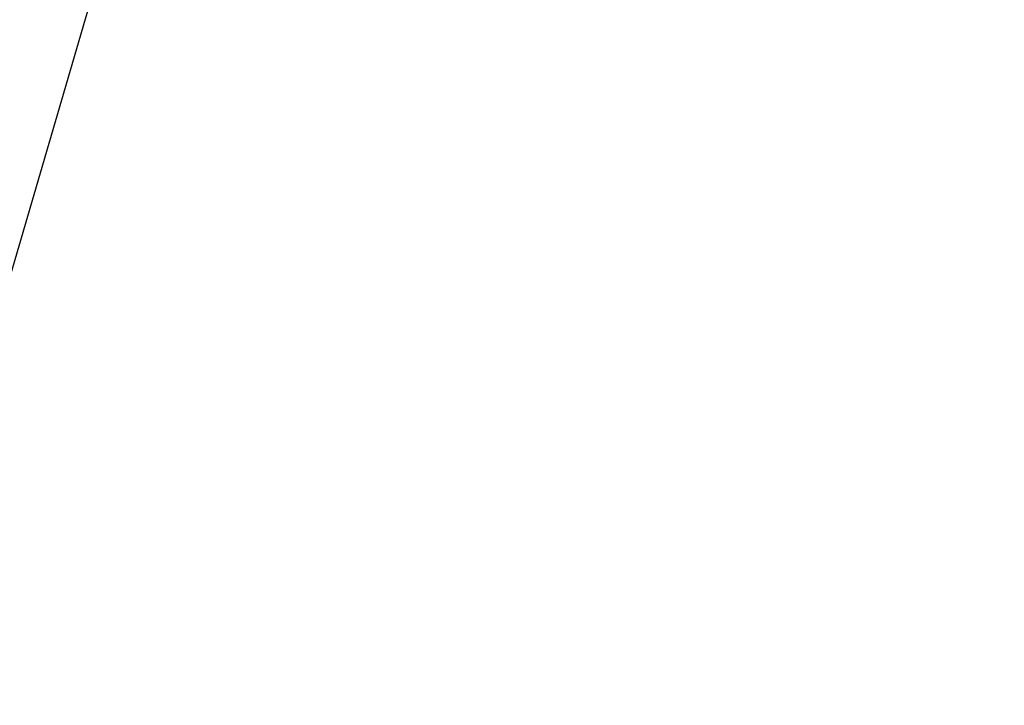
# Model space of a CAD drawing. Units: inches. Extents: x 3590 to 5167, y 65 to 1917.
# Tile 92 of 100: x 5052.8768 to 5053.476, y 1788.6144 to 1789.0318. Entities that reach past the tile are written whole.
import ezdxf

# ---------------------------------------------------------------- set-up
doc = ezdxf.new("R2010")
doc.units = ezdxf.units.IN
for name, color, linetype, lineweight in [('A-ANNO-DIMS', 2, 'Continuous', 18), ('A-FLOR-PATT', 8, 'Continuous', 13), ('L-PLNT', 94, 'Continuous', 18)]:
    doc.layers.add(name, color=color, linetype=linetype, lineweight=lineweight)
doc.layers.add('DIENHOA', color=3, linetype='Continuous')
doc.styles.get("Standard").update_dxf_attribs({"font": 'arial.ttf'})
doc.dimstyles.new('ISO-25', dxfattribs={"dimtxt": 9, "dimasz": 2.5, "dimexe": 1.25, "dimexo": 0.625, "dimtad": 1, "dimdec": 1, "dimlunit": 3, "dimtxsty": 'Standard', "dimcen": 2.5, "dimadec": 0, "dimazin": 0, "dimtfac": 1, "dimtdec": 1, "dimtmove": 0, "dimatfit": 3, "dimfxl": 1, "dimarcsym": 0})

# ---------------------------------------------------------------- blocks, each defined once
blk = doc.blocks.new('Cay03_mb')
at = {"layer": 'DIENHOA'}
blk.add_line((118.956, 441.661), (96.72, 365.576), dxfattribs=at)
blk = doc.blocks.new('*D323')
at = {"layer": 'A-ANNO-DIMS', "color": 0, "lineweight": -2, "transparency": 16777216}
for p, q in [((5069.17227, 1795.21603), (5069.17227, 1874.95034)), ((5065.43703, 1795.21603), (5070.42227, 1795.21603)), ((5069.17227, 1769.30924), (5069.17227, 1792.71603)), ((5065.43703, 1766.80924), (5070.42227, 1766.80924))]:
    blk.add_line(p, q, dxfattribs=at)
at = {"layer": 'A-ANNO-DIMS', "color": 0, "transparency": 16777216}
for points in [[(5068.75561, 1792.71603), (5069.58894, 1792.71603), (5069.17227, 1795.21603)], [(5068.75561, 1769.30924), (5069.58894, 1769.30924), (5069.17227, 1766.80924)]]:
    blk.add_solid(points, dxfattribs=at)
at = {"layer": 'Defpoints', "color": 0, "transparency": 16777216}
for p in [(5064.81203, 1795.21603), (5069.17227, 1795.21603), (5064.81203, 1766.80924)]:
    blk.add_point(p, dxfattribs=at)
at = {"layer": 'A-ANNO-DIMS', "color": 0, "transparency": 16777216, "insert": (5063.89379, 1836.33318), "char_height": 9, "attachment_point": 5, "rotation": 90}
blk.add_mtext('2\'-4 1/2" TYP.', dxfattribs=at)

msp = doc.modelspace()

# ---------------------------------------------------------------- hatches: boundary and pattern name
at = {"layer": 'A-FLOR-PATT', "transparency": 33554687}
h = msp.add_hatch(dxfattribs=at)
h.set_pattern_fill('AR-HBONE', color=256, scale=0.2)
h.set_pattern_definition([(45, (-588.972, 0), (0, 28.73682), [60.96, -20.32]), (135, (-574.604, 14.368), (3e-15, 28.73682), [60.96, -20.32])])
h.paths.add_polyline_path([(5071.27403, 1796.99898), (4933.27403, 1796.99898), (4933.27403, 1753.99898), (4962.77403, 1753.99898, -0.414214), (4928.77403, 1719.99898), (4933.27403, 1718.99898), (4933.27403, 1334.99898), (5071.27403, 1334.99898)])
h.paths.add_polyline_path([(4951.78002, 1521.0767), (4951.7151, 1521.0404), (4951.56345, 1520.89532)], flags=16)
h.paths.add_polyline_path([(4952.267, 1521.37645), (4952.1977, 1521.37111), (4952.19823, 1521.35558)], flags=0)
h.paths.add_polyline_path([(4967.05076, 1529.72832), (4965.23122, 1528.69444), (4963.41109, 1527.71401), (4961.75649, 1526.85081), (4963.58887, 1527.44938), (4964.03555, 1527.47802), (4962.9755, 1527.24902), (4961.76022, 1526.85203), (4959.79219, 1525.83406), (4958.00498, 1524.89483), (4956.24031, 1523.92961), (4954.50395, 1522.91854), (4954.1294, 1522.68163), (4953.36051, 1521.99688), (4953.36558, 1521.99754), (4953.605, 1522.06367), (4955.10605, 1522.76083), (4956.92108, 1523.43405), (4958.67784, 1523.91513), (4960.35834, 1524.20036), (4961.94456, 1524.28606), (4964.17144, 1524.10849), (4965.95752, 1523.30903), (4963.86273, 1522.97565), (4965.18742, 1522.49898), (4963.36614, 1522.49715), (4961.54526, 1522.48682), (4959.76359, 1522.46077), (4958.30414, 1522.4188), (4957.97356, 1522.38829), (4956.30692, 1522.2324), (4954.71821, 1522.07143), (4953.25077, 1521.89915), (4953.52509, 1521.62277), (4954.33087, 1521.37883), (4956.24263, 1521.22987), (4958.03913, 1520.92952), (4959.68424, 1520.48339), (4961.16007, 1519.89569), (4963.10699, 1518.80022), (4964.39286, 1517.32518), (4962.97306, 1517.72596), (4964.55841, 1516.66059), (4965.40664, 1515.70779), (4963.50733, 1516.32179), (4961.67995, 1517.0051), (4959.93478, 1517.74489), (4958.2821, 1518.52833), (4956.73216, 1519.34257), (4955.29527, 1520.17478), (4954.67155, 1520.57237), (4954.51279, 1520.6271), (4955.65848, 1519.31837), (4956.70263, 1517.98232), (4957.64403, 1516.64663), (4958.48545, 1515.33439), (4959.54998, 1513.52398), (4960.43768, 1511.76936), (4958.84107, 1513.6196), (4957.45175, 1515.3249), (4955.8186, 1517.45855), (4956.66537, 1515.44764), (4957.11109, 1513.92292), (4957.44681, 1511.71434), (4957.07641, 1509.79288), (4956.53757, 1511.1103), (4955.99231, 1512.56892), (4955.44448, 1514.12509), (4954.89794, 1515.73518), (4954.35653, 1517.35553), (4953.82412, 1518.94251), (4953.30455, 1520.45247), (4953.06452, 1521.11563), (4952.97143, 1521.14607), (4952.94932, 1521.08646), (4952.72981, 1520.19905), (4953.3698, 1518.02364), (4953.75708, 1516.37279), (4954.05124, 1514.76538), (4954.26449, 1513.22121), (4954.47124, 1511.13121), (4954.4971, 1510.40174), (4954.40903, 1511.76006), (4954.26449, 1513.22121), (4954.05124, 1514.76538), (4953.75708, 1516.37279), (4953.3698, 1518.02364), (4952.87718, 1519.69813), (4952.7161, 1520.1412), (4952.53301, 1519.05871), (4952.37428, 1517.78881), (4952.21925, 1516.31167), (4952.04598, 1514.59986), (4951.83253, 1512.62598), (4951.55697, 1510.36259), (4951.20331, 1512.16818), (4950.85168, 1514.33931), (4950.98529, 1516.37594), (4951.6596, 1518.28625), (4952.59261, 1520.48085), (4952.35664, 1521.1299), (4951.85502, 1520.32753), (4950.83901, 1518.90828), (4949.77675, 1517.58658), (4948.91554, 1516.61731), (4948.11099, 1515.2561), (4947.0891, 1513.55389), (4945.88937, 1511.61495), (4946.32587, 1513.40232), (4946.5624, 1514.24913), (4945.52771, 1513.32668), (4944.58105, 1512.53126), (4946.01774, 1514.50825), (4947.2044, 1516.04763), (4947.89331, 1517.31331), (4949.30686, 1518.76446), (4950.41417, 1519.76716), (4950.45131, 1519.80628), (4952.267, 1521.37645), (4951.64457, 1521.49317), (4950.40371, 1521.17954), (4948.04447, 1520.35868), (4946.11863, 1519.45198), (4944.57182, 1518.47484), (4943.34962, 1517.44265), (4941.99695, 1515.91971), (4941.66146, 1515.27475), (4942.81332, 1516.98973), (4944.57182, 1518.47484), (4946.11863, 1519.45198), (4948.04447, 1520.35868), (4950.40371, 1521.17954), (4951.64457, 1521.49317), (4949.64678, 1521.86781), (4948.59979, 1521.75633), (4947.12629, 1521.5699), (4945.42015, 1521.34763), (4943.44969, 1521.10462), (4941.18319, 1520.85596), (4942.86028, 1521.61265), (4943.87308, 1522.03014), (4942.95216, 1521.9093), (4941.40968, 1521.48512), (4939.54287, 1520.67019), (4938.96775, 1520.2255), (4940.73284, 1521.29899), (4942.95216, 1521.9093), (4943.70184, 1522.00767), (4945.89419, 1522.69998), (4947.56488, 1522.71399), (4948.92086, 1522.56573), (4951.13144, 1522.18271), (4950.97062, 1522.2969), (4948.12924, 1523.00563), (4946.03496, 1523.70671), (4944.23235, 1524.52143), (4942.70692, 1525.46111), (4941.44419, 1526.53707), (4940.42968, 1527.76062), (4939.6489, 1529.14306), (4941.42091, 1528.12232), (4943.14742, 1527.13248), (4944.84093, 1526.17457), (4946.51394, 1525.24959), (4948.17893, 1524.35855), (4948.36457, 1524.26336), (4946.47531, 1526.04459), (4945.18083, 1527.54042), (4944.19039, 1529.03339), (4943.49559, 1530.53985), (4943.27808, 1531.3597), (4942.49849, 1531.91903), (4943.11353, 1531.76249), (4942.95927, 1533.6586), (4944.13953, 1531.9886), (4944.61171, 1531.32339), (4946.20163, 1530.46341), (4947.48567, 1529.50925), (4948.79027, 1528.22649), (4950.36754, 1526.23746), (4949.48547, 1528.15549), (4948.85128, 1530.12254), (4948.49054, 1532.04127), (4948.38105, 1533.91822), (4948.50062, 1535.7599), (4948.82704, 1537.57284), (4949.41803, 1535.56526), (4949.95684, 1533.56932), (4950.46414, 1531.5861), (4950.96058, 1529.6167), (4951.3911, 1527.95448), (4951.72352, 1530.68689), (4952.20106, 1532.57994), (4952.88914, 1534.32964), (4953.77035, 1535.95123), (4954.82726, 1537.45995), (4954.52145, 1535.38966), (4954.27314, 1533.93684), (4955.57999, 1535.6627), (4956.74758, 1536.73859), (4956.15852, 1534.78029), (4955.58917, 1532.87334), (4955.04336, 1531.00581), (4954.52493, 1529.16576), (4954.03771, 1527.34127), (4953.63833, 1525.73298), (4953.61143, 1525.58564), (4953.39805, 1524.16565), (4953.38219, 1524.00887), (4954.06955, 1525.47563), (4954.91212, 1527.02173), (4956.13627, 1528.89351), (4957.84668, 1530.57701), (4959.37601, 1531.54014), (4958.25596, 1530.10398), (4957.14284, 1528.66291), (4956.06626, 1527.24305), (4955.05579, 1525.87054), (4954.14104, 1524.57149), (4953.35159, 1523.37204), (4953.31079, 1523.30299), (4953.27253, 1522.92478), (4953.26102, 1522.38213), (4954.1031, 1523.37273), (4954.63005, 1524.28376), (4955.96149, 1526.35767), (4957.23002, 1528.12969), (4958.42057, 1529.60864), (4960.03671, 1531.36792), (4961.3736, 1532.3752), (4962.1015, 1532.77), (4961.06994, 1531.06113), (4959.98733, 1529.43811), (4958.86851, 1527.90803), (4958.15046, 1527.00742), (4959.80291, 1528.00314), (4961.58854, 1528.79257), (4963.39087, 1529.32783), (4965.21118, 1529.63205)], flags=16)
h.paths.add_polyline_path([(4962.94387, 1523.18187), (4961.10714, 1523.42192), (4960.39205, 1523.36158), (4962.34964, 1523.33061)], flags=0)
h.paths.add_polyline_path([(5049.54129, 1584.55089), (5049.47636, 1584.51458), (5049.32471, 1584.3695)], flags=16)
h.paths.add_polyline_path([(5050.02827, 1584.85063), (5049.95897, 1584.84529), (5049.95949, 1584.82976)], flags=0)
h.paths.add_polyline_path([(5042.33308, 1581.94902), (5043.8799, 1582.92616), (5045.80573, 1583.83286), (5048.16498, 1584.65372), (5049.40583, 1584.96736), (5047.40804, 1585.34199), (5046.36106, 1585.23052), (5044.88755, 1585.04408), (5043.18142, 1584.82181), (5041.21095, 1584.5788), (5038.94446, 1584.33014), (5040.62155, 1585.08683), (5041.63434, 1585.50432), (5040.71343, 1585.38348), (5039.17095, 1584.9593), (5037.30414, 1584.14438), (5036.72901, 1583.69969), (5038.4941, 1584.77317), (5040.71343, 1585.38348), (5041.4631, 1585.48185), (5043.65545, 1586.17416), (5045.32615, 1586.18818), (5046.68212, 1586.03992), (5048.8927, 1585.6569), (5048.73188, 1585.77108), (5045.89051, 1586.47981), (5043.79622, 1587.18089), (5041.99361, 1587.99561), (5040.46818, 1588.9353), (5039.20546, 1590.01125), (5038.19095, 1591.2348), (5037.41016, 1592.61725), (5039.18217, 1591.5965), (5040.90868, 1590.60667), (5042.6022, 1589.64876), (5044.2752, 1588.72378), (5045.94019, 1587.83274), (5046.12584, 1587.73754), (5044.23658, 1589.51878), (5042.9421, 1591.01461), (5041.95166, 1592.50757), (5041.25685, 1594.01403), (5041.03935, 1594.83388), (5040.25976, 1595.39321), (5040.8748, 1595.23667), (5040.72054, 1597.13279), (5041.9008, 1595.46278), (5042.37297, 1594.79758), (5043.96289, 1593.93759), (5045.24694, 1592.98344), (5046.55153, 1591.70068), (5048.12881, 1589.71164), (5047.24673, 1591.62967), (5046.61254, 1593.59672), (5046.2518, 1595.51546), (5046.14232, 1597.3924), (5046.26189, 1599.23408), (5046.5883, 1601.04703), (5047.17929, 1599.03944), (5047.71811, 1597.0435), (5048.22541, 1595.06028), (5048.72184, 1593.09089), (5049.15237, 1591.42866), (5049.48478, 1594.16107), (5049.96233, 1596.05412), (5050.65041, 1597.80382), (5051.53161, 1599.42541), (5052.58852, 1600.93414), (5052.28271, 1598.86384), (5052.03441, 1597.41102), (5053.34126, 1599.13689), (5054.50884, 1600.21277), (5053.91979, 1598.25447), (5053.35044, 1596.34752), (5052.80463, 1594.47999), (5052.2862, 1592.63995), (5051.79898, 1590.81546), (5051.39959, 1589.20716), (5051.3727, 1589.05983), (5051.15931, 1587.63984), (5051.14346, 1587.48305), (5051.83082, 1588.94982), (5052.67339, 1590.49592), (5053.89754, 1592.3677), (5055.60794, 1594.05119), (5057.13728, 1595.01432), (5056.01722, 1593.57817), (5054.90411, 1592.1371), (5053.82752, 1590.71724), (5052.81705, 1589.34472), (5051.9023, 1588.04567), (5051.11286, 1586.84622), (5051.07205, 1586.77718), (5051.03379, 1586.39896), (5051.02228, 1585.85631), (5051.86437, 1586.84692), (5052.39131, 1587.75794), (5053.72275, 1589.83185), (5054.99128, 1591.60387), (5056.18183, 1593.08282), (5057.79798, 1594.84211), (5059.13486, 1595.84938), (5059.86276, 1596.24419), (5058.83121, 1594.53531), (5057.7486, 1592.9123), (5056.62978, 1591.38221), (5055.91173, 1590.4816), (5057.56418, 1591.47732), (5059.34981, 1592.26675), (5061.15214, 1592.80202), (5062.97245, 1593.10624), (5064.81203, 1593.20251), (5062.99248, 1592.16863), (5061.17235, 1591.18819), (5059.51775, 1590.325), (5061.35014, 1590.92356), (5061.79682, 1590.95221), (5060.73676, 1590.7232), (5059.52148, 1590.32622), (5057.55345, 1589.30825), (5055.76625, 1588.36901), (5054.00157, 1587.40379), (5052.26521, 1586.39273), (5051.89067, 1586.15581), (5051.12177, 1585.47106), (5051.12684, 1585.47172), (5051.36627, 1585.53786), (5052.86732, 1586.23502), (5054.68234, 1586.90824), (5056.4391, 1587.38931), (5058.1196, 1587.67454), (5059.70582, 1587.76024), (5061.93271, 1587.58268), (5063.71878, 1586.78321), (5061.62399, 1586.44983), (5062.94869, 1585.97317), (5061.12741, 1585.97133), (5059.30653, 1585.961), (5057.52486, 1585.93496), (5056.06541, 1585.89299), (5055.73482, 1585.86247), (5054.06819, 1585.70658), (5052.47947, 1585.54561), (5051.01204, 1585.37333), (5051.28635, 1585.09695), (5052.09214, 1584.85301), (5054.00389, 1584.70406), (5055.8004, 1584.4037), (5057.44551, 1583.95757), (5058.92133, 1583.36987), (5060.86825, 1582.27441), (5062.15413, 1580.79937), (5060.73433, 1581.20015), (5062.31967, 1580.13477), (5063.1679, 1579.18198), (5061.2686, 1579.79597), (5059.44122, 1580.47928), (5057.69605, 1581.21908), (5056.04336, 1582.00251), (5054.49343, 1582.81675), (5053.05653, 1583.64897), (5052.43281, 1584.04656), (5052.27405, 1584.10128), (5053.41974, 1582.79255), (5054.4639, 1581.4565), (5055.40529, 1580.12081), (5056.24672, 1578.80858), (5057.31125, 1576.99816), (5058.19895, 1575.24354), (5056.60234, 1577.09378), (5055.21301, 1578.79908), (5053.57987, 1580.93274), (5054.42664, 1578.92183), (5054.87235, 1577.3971), (5055.20808, 1575.18852), (5054.83767, 1573.26706), (5054.29883, 1574.58448), (5053.75357, 1576.0431), (5053.20575, 1577.59927), (5052.6592, 1579.20936), (5052.1178, 1580.82971), (5051.58538, 1582.41669), (5051.06582, 1583.92666), (5050.82578, 1584.58981), (5050.7327, 1584.62025), (5050.71058, 1584.56064), (5050.49108, 1583.67323), (5051.13107, 1581.49782), (5051.51835, 1579.84698), (5051.8125, 1578.23957), (5052.02575, 1576.69539), (5052.23251, 1574.6054), (5052.25836, 1573.87593), (5052.1703, 1575.23424), (5052.02575, 1576.69539), (5051.8125, 1578.23957), (5051.51835, 1579.84698), (5051.13107, 1581.49782), (5050.63844, 1583.17231), (5050.47736, 1583.61538), (5050.29428, 1582.53289), (5050.13554, 1581.26299), (5049.98051, 1579.78585), (5049.80724, 1578.07405), (5049.59379, 1576.10016), (5049.31823, 1573.83678), (5048.96458, 1575.64237), (5048.61294, 1577.8135), (5048.74656, 1579.85012), (5049.42086, 1581.76043), (5050.35388, 1583.95503), (5050.1179, 1584.60408), (5049.61629, 1583.80172), (5048.60027, 1582.38246), (5047.53801, 1581.06076), (5046.67681, 1580.09149), (5045.87225, 1578.73029), (5044.85036, 1577.02808), (5043.65063, 1575.08913), (5044.08713, 1576.8765), (5044.32366, 1577.72331), (5043.28898, 1576.80086), (5042.34232, 1576.00545), (5043.779, 1577.98243), (5044.96566, 1579.52182), (5045.65457, 1580.78749), (5047.06813, 1582.23865), (5048.17543, 1583.24134), (5048.21258, 1583.28047), (5050.02827, 1584.85063), (5049.40583, 1584.96736), (5048.16498, 1584.65372), (5045.80573, 1583.83286), (5043.8799, 1582.92616), (5042.33308, 1581.94902), (5041.11088, 1580.91684), (5039.75821, 1579.39389), (5039.42272, 1578.74894), (5040.57458, 1580.46391)], flags=16)
h.paths.add_polyline_path([(4954.79872, 1533.12029), (4954.26249, 1532.07935), (4953.83112, 1530.93464), (4953.50472, 1529.63602), (4953.28338, 1528.13331), (4953.16721, 1526.37637), (4953.15631, 1524.31504), (4953.27669, 1521.23629), (4952.80168, 1521.84177), (4951.55695, 1521.99789), (4950.97575, 1521.9613), (4952.66059, 1521.94097), (4952.80168, 1521.84177), (4953.15249, 1523.59258), (4953.16721, 1526.37637), (4953.28338, 1528.13331), (4953.60929, 1530.34598), (4954.45558, 1532.59174)], flags=0)
h.paths.add_polyline_path([(5050.56294, 1585.31596), (5049.31822, 1585.47208), (5048.73702, 1585.43548), (5050.42186, 1585.41516), (5050.56294, 1585.31596), (5050.91375, 1587.06676), (5050.92848, 1589.85056), (5051.04465, 1591.6075), (5051.37055, 1593.82017), (5052.21684, 1596.06593), (5052.55999, 1596.59447), (5052.02375, 1595.55353), (5051.59238, 1594.40883), (5051.26598, 1593.1102), (5051.04465, 1591.6075), (5050.92848, 1589.85056), (5050.91757, 1587.78922), (5051.03795, 1584.71048)], flags=0)
h.paths.add_polyline_path([(5058.15332, 1586.83576), (5060.11091, 1586.80479), (5060.70514, 1586.65605), (5058.8684, 1586.8961)], flags=0)
h.paths.add_polyline_path([(5049.54129, 1430.93611), (5049.47636, 1430.8998), (5049.32471, 1430.75472)], flags=16)
h.paths.add_polyline_path([(5050.02827, 1431.23585), (5049.95897, 1431.23051), (5049.95949, 1431.21498)], flags=0)
h.paths.add_polyline_path([(5046.5883, 1447.43225), (5047.17929, 1445.42467), (5047.71811, 1443.42872), (5048.22541, 1441.4455), (5048.72184, 1439.47611), (5049.15237, 1437.81388), (5049.48478, 1440.5463), (5049.96233, 1442.43934), (5050.65041, 1444.18904), (5051.53161, 1445.81063), (5052.58852, 1447.31936), (5052.28271, 1445.24906), (5052.03441, 1443.79624), (5053.34126, 1445.52211), (5054.50884, 1446.59799), (5053.91979, 1444.63969), (5053.35044, 1442.73274), (5052.80463, 1440.86521), (5052.2862, 1439.02517), (5051.79898, 1437.20068), (5051.39959, 1435.59238), (5051.3727, 1435.44505), (5051.15931, 1434.02506), (5051.14346, 1433.86828), (5051.83082, 1435.33504), (5052.67339, 1436.88114), (5053.89754, 1438.75292), (5055.60794, 1440.43641), (5057.13728, 1441.39954), (5056.01722, 1439.96339), (5054.90411, 1438.52232), (5053.82752, 1437.10246), (5052.81705, 1435.72994), (5051.9023, 1434.4309), (5051.11286, 1433.23145), (5051.07205, 1433.1624), (5051.03379, 1432.78418), (5051.02228, 1432.24153), (5051.86437, 1433.23214), (5052.39131, 1434.14316), (5053.72275, 1436.21707), (5054.99128, 1437.98909), (5056.18183, 1439.46805), (5057.79798, 1441.22733), (5059.13486, 1442.23461), (5059.86276, 1442.62941), (5058.83121, 1440.92053), (5057.7486, 1439.29752), (5056.62978, 1437.76743), (5055.91173, 1436.86682), (5057.56418, 1437.86255), (5059.34981, 1438.65197), (5061.15214, 1439.18724), (5062.97245, 1439.49146), (5064.81203, 1439.58773), (5062.99248, 1438.55385), (5061.17235, 1437.57342), (5059.51775, 1436.71022), (5061.35014, 1437.30879), (5061.79682, 1437.33743), (5060.73676, 1437.10842), (5059.52148, 1436.71144), (5057.55345, 1435.69347), (5055.76625, 1434.75423), (5054.00157, 1433.78901), (5052.26521, 1432.77795), (5051.89067, 1432.54103), (5051.12177, 1431.85628), (5051.12684, 1431.85694), (5051.36627, 1431.92308), (5052.86732, 1432.62024), (5054.68234, 1433.29346), (5056.4391, 1433.77453), (5058.1196, 1434.05976), (5059.70582, 1434.14546), (5061.93271, 1433.9679), (5063.71878, 1433.16843), (5061.62399, 1432.83505), (5062.94869, 1432.35839), (5061.12741, 1432.35655), (5059.30653, 1432.34623), (5057.52486, 1432.32018), (5056.06541, 1432.27821), (5055.73482, 1432.24769), (5054.06819, 1432.09181), (5052.47947, 1431.93083), (5051.01204, 1431.75856), (5051.28635, 1431.48218), (5052.09214, 1431.23823), (5054.00389, 1431.08928), (5055.8004, 1430.78892), (5057.44551, 1430.34279), (5058.92133, 1429.75509), (5060.86825, 1428.65963), (5062.15413, 1427.18459), (5060.73433, 1427.58537), (5062.31967, 1426.52), (5063.1679, 1425.5672), (5061.2686, 1426.18119), (5059.44122, 1426.86451), (5057.69605, 1427.6043), (5056.04336, 1428.38773), (5054.49343, 1429.20197), (5053.05653, 1430.03419), (5052.43281, 1430.43178), (5052.27405, 1430.48651), (5053.41974, 1429.17777), (5054.4639, 1427.84172), (5055.40529, 1426.50603), (5056.24672, 1425.1938), (5057.31125, 1423.38338), (5058.19895, 1421.62877), (5056.60234, 1423.479), (5055.21301, 1425.1843), (5053.57987, 1427.31796), (5054.42664, 1425.30705), (5054.87235, 1423.78233), (5055.20808, 1421.57374), (5054.83767, 1419.65228), (5054.29883, 1420.9697), (5053.75357, 1422.42832), (5053.20575, 1423.9845), (5052.6592, 1425.59458), (5052.1178, 1427.21493), (5051.58538, 1428.80191), (5051.06582, 1430.31188), (5050.82578, 1430.97503), (5050.7327, 1431.00547), (5050.71058, 1430.94586), (5050.49108, 1430.05845), (5051.13107, 1427.88305), (5051.51835, 1426.2322), (5051.8125, 1424.62479), (5052.02575, 1423.08061), (5052.23251, 1420.99062), (5052.25836, 1420.26115), (5052.1703, 1421.61947), (5052.02575, 1423.08061), (5051.8125, 1424.62479), (5051.51835, 1426.2322), (5051.13107, 1427.88305), (5050.63844, 1429.55753), (5050.47736, 1430.0006), (5050.29428, 1428.91811), (5050.13554, 1427.64821), (5049.98051, 1426.17107), (5049.80724, 1424.45927), (5049.59379, 1422.48539), (5049.31823, 1420.222), (5048.96458, 1422.02759), (5048.61294, 1424.19872), (5048.74656, 1426.23534), (5049.42086, 1428.14565), (5050.35388, 1430.34025), (5050.1179, 1430.98931), (5049.61629, 1430.18694), (5048.60027, 1428.76768), (5047.53801, 1427.44598), (5046.67681, 1426.47671), (5045.87225, 1425.11551), (5044.85036, 1423.4133), (5043.65063, 1421.47435), (5044.08713, 1423.26172), (5044.32366, 1424.10854), (5043.28898, 1423.18608), (5042.34232, 1422.39067), (5043.779, 1424.36765), (5044.96566, 1425.90704), (5045.65457, 1427.17272), (5047.06813, 1428.62387), (5048.17543, 1429.62657), (5048.21258, 1429.66569), (5050.02827, 1431.23585), (5049.40583, 1431.35258), (5048.16498, 1431.03894), (5045.80573, 1430.21809), (5043.8799, 1429.31139), (5042.33308, 1428.33424), (5041.11088, 1427.30206), (5039.75821, 1425.77911), (5039.42272, 1425.13416), (5040.57458, 1426.84914), (5042.33308, 1428.33424), (5043.8799, 1429.31139), (5045.80573, 1430.21809), (5048.16498, 1431.03894), (5049.40583, 1431.35258), (5047.40804, 1431.72722), (5046.36106, 1431.61574), (5044.88755, 1431.42931), (5043.18142, 1431.20704), (5041.21095, 1430.96402), (5038.94446, 1430.71536), (5040.62155, 1431.47205), (5041.63434, 1431.88954), (5040.71343, 1431.76871), (5039.17095, 1431.34453), (5037.30414, 1430.5296), (5036.72901, 1430.08491), (5038.4941, 1431.1584), (5040.71343, 1431.76871), (5041.4631, 1431.86707), (5043.65545, 1432.55939), (5045.32615, 1432.5734), (5046.68212, 1432.42514), (5048.8927, 1432.04212), (5048.73188, 1432.1563), (5045.89051, 1432.86503), (5043.79622, 1433.56611), (5041.99361, 1434.38083), (5040.46818, 1435.32052), (5039.20546, 1436.39648), (5038.19095, 1437.62002), (5037.41016, 1439.00247), (5039.18217, 1437.98172), (5040.90868, 1436.99189), (5042.6022, 1436.03398), (5044.2752, 1435.109), (5045.94019, 1434.21796), (5046.12584, 1434.12276), (5044.23658, 1435.904), (5042.9421, 1437.39983), (5041.95166, 1438.8928), (5041.25685, 1440.39925), (5041.03935, 1441.2191), (5040.25976, 1441.77844), (5040.8748, 1441.62189), (5040.72054, 1443.51801), (5041.9008, 1441.848), (5042.37297, 1441.1828), (5043.96289, 1440.32282), (5045.24694, 1439.36866), (5046.55153, 1438.0859), (5048.12881, 1436.09686), (5047.24673, 1438.01489), (5046.61254, 1439.98195), (5046.2518, 1441.90068), (5046.14232, 1443.77762), (5046.26189, 1445.6193)], flags=16)
h.paths.add_polyline_path([(5052.38176, 1444.25496), (5051.62263, 1442.77987), (5052.02375, 1441.93875), (5052.55999, 1442.9797)], flags=0)
h.paths.add_polyline_path([(5050.56294, 1431.70118), (5049.31822, 1431.8573), (5048.73702, 1431.82071), (5050.42186, 1431.80038)], flags=0)
h.paths.add_polyline_path([(5058.15332, 1433.22098), (5060.11091, 1433.19001), (5060.70514, 1433.04127), (5058.8684, 1433.28132)], flags=0)
h.paths.add_polyline_path([(5049.54129, 1352.28535), (5049.47636, 1352.24904), (5049.32471, 1352.10396)], flags=16)
h.paths.add_polyline_path([(5050.02827, 1352.58509), (5049.95897, 1352.57975), (5049.95949, 1352.56422)], flags=0)
h.paths.add_polyline_path([(5046.5883, 1368.78149), (5047.17929, 1366.7739), (5047.71811, 1364.77796), (5048.22541, 1362.79474), (5048.72184, 1360.82534), (5049.15237, 1359.16312), (5049.48478, 1361.89553), (5049.96233, 1363.78858), (5050.65041, 1365.53828), (5051.53161, 1367.15987), (5052.58852, 1368.6686), (5052.28271, 1366.5983), (5052.03441, 1365.14548), (5053.34126, 1366.87135), (5054.50884, 1367.94723), (5053.91979, 1365.98893), (5053.35044, 1364.08198), (5052.80463, 1362.21445), (5052.2862, 1360.37441), (5051.79898, 1358.54992), (5051.39959, 1356.94162), (5051.3727, 1356.79428), (5051.15931, 1355.37429), (5051.14346, 1355.21751), (5051.83082, 1356.68428), (5052.67339, 1358.23037), (5053.89754, 1360.10216), (5055.60794, 1361.78565), (5057.13728, 1362.74878), (5056.01722, 1361.31262), (5054.90411, 1359.87155), (5053.82752, 1358.4517), (5052.81705, 1357.07918), (5051.9023, 1355.78013), (5051.11286, 1354.58068), (5051.07205, 1354.51164), (5051.03379, 1354.13342), (5051.02228, 1353.59077), (5051.86437, 1354.58137), (5052.39131, 1355.4924), (5053.72275, 1357.56631), (5054.99128, 1359.33833), (5056.18183, 1360.81728), (5057.79798, 1362.57656), (5059.13486, 1363.58384), (5059.86276, 1363.97864), (5058.83121, 1362.26977), (5057.7486, 1360.64675), (5056.62978, 1359.11667), (5055.91173, 1358.21606), (5057.56418, 1359.21178), (5059.34981, 1360.00121), (5061.15214, 1360.53648), (5062.97245, 1360.84069), (5064.81203, 1360.93697), (5062.99248, 1359.90308), (5061.17235, 1358.92265), (5059.51775, 1358.05946), (5061.35014, 1358.65802), (5061.79682, 1358.68666), (5060.73676, 1358.45766), (5059.52148, 1358.06068), (5057.55345, 1357.0427), (5055.76625, 1356.10347), (5054.00157, 1355.13825), (5052.26521, 1354.12718), (5051.89067, 1353.89027), (5051.12177, 1353.20552), (5051.12684, 1353.20618), (5051.36627, 1353.27231), (5052.86732, 1353.96947), (5054.68234, 1354.6427), (5056.4391, 1355.12377), (5058.1196, 1355.409), (5059.70582, 1355.4947), (5061.93271, 1355.31713), (5063.71878, 1354.51767), (5061.62399, 1354.18429), (5062.94869, 1353.70763), (5061.12741, 1353.70579), (5059.30653, 1353.69546), (5057.52486, 1353.66942), (5056.06541, 1353.62744), (5055.73482, 1353.59693), (5054.06819, 1353.44104), (5052.47947, 1353.28007), (5051.01204, 1353.10779), (5051.28635, 1352.83141), (5052.09214, 1352.58747), (5054.00389, 1352.43852), (5055.8004, 1352.13816), (5057.44551, 1351.69203), (5058.92133, 1351.10433), (5060.86825, 1350.00887), (5062.15413, 1348.53382), (5060.73433, 1348.9346), (5062.31967, 1347.86923), (5063.1679, 1346.91643), (5061.2686, 1347.53043), (5059.44122, 1348.21374), (5057.69605, 1348.95353), (5056.04336, 1349.73697), (5054.49343, 1350.55121), (5053.05653, 1351.38342), (5052.43281, 1351.78101), (5052.27405, 1351.83574), (5053.41974, 1350.52701), (5054.4639, 1349.19096), (5055.40529, 1347.85527), (5056.24672, 1346.54303), (5057.31125, 1344.73262), (5058.19895, 1342.978), (5056.60234, 1344.82824), (5055.21301, 1346.53354), (5053.57987, 1348.6672), (5054.42664, 1346.65629), (5054.87235, 1345.13156), (5055.20808, 1342.92298), (5054.83767, 1341.00152), (5054.29883, 1342.31894), (5053.75357, 1343.77756), (5053.20575, 1345.33373), (5052.6592, 1346.94382), (5052.1178, 1348.56417), (5051.58538, 1350.15115), (5051.06582, 1351.66111), (5050.82578, 1352.32427), (5050.7327, 1352.35471), (5050.71058, 1352.2951), (5050.49108, 1351.40769), (5051.13107, 1349.23228), (5051.51835, 1347.58144), (5051.8125, 1345.97403), (5052.02575, 1344.42985), (5052.23251, 1342.33986), (5052.25836, 1341.61039), (5052.1703, 1342.9687), (5052.02575, 1344.42985), (5051.8125, 1345.97403), (5051.51835, 1347.58144), (5051.13107, 1349.23228), (5050.63844, 1350.90677), (5050.47736, 1351.34984), (5050.29428, 1350.26735), (5050.13554, 1348.99745), (5049.98051, 1347.52031), (5049.80724, 1345.80851), (5049.59379, 1343.83462), (5049.31823, 1341.57124), (5048.96458, 1343.37683), (5048.61294, 1345.54796), (5048.74656, 1347.58458), (5049.42086, 1349.49489), (5050.35388, 1351.68949), (5050.1179, 1352.33854), (5049.61629, 1351.53617), (5048.60027, 1350.11692), (5047.53801, 1348.79522), (5046.67681, 1347.82595), (5045.87225, 1346.46475), (5044.85036, 1344.76253), (5043.65063, 1342.82359), (5044.08713, 1344.61096), (5044.32366, 1345.45777), (5043.28898, 1344.53532), (5042.34232, 1343.7399), (5043.779, 1345.71689), (5044.96566, 1347.25627), (5045.65457, 1348.52195), (5047.06813, 1349.9731), (5048.17543, 1350.9758), (5048.21258, 1351.01493), (5050.02827, 1352.58509), (5049.40583, 1352.70181), (5048.16498, 1352.38818), (5045.80573, 1351.56732), (5043.8799, 1350.66062), (5042.33308, 1349.68348), (5041.11088, 1348.65129), (5039.75821, 1347.12835), (5039.42272, 1346.4834), (5040.57458, 1348.19837), (5042.33308, 1349.68348), (5043.8799, 1350.66062), (5045.80573, 1351.56732), (5048.16498, 1352.38818), (5049.40583, 1352.70181), (5047.40804, 1353.07645), (5046.36106, 1352.96498), (5044.88755, 1352.77854), (5043.18142, 1352.55627), (5041.21095, 1352.31326), (5038.94446, 1352.0646), (5040.62155, 1352.82129), (5041.63434, 1353.23878), (5040.71343, 1353.11794), (5039.17095, 1352.69376), (5037.30414, 1351.87884), (5036.72901, 1351.43415), (5038.4941, 1352.50763), (5040.71343, 1353.11794), (5041.4631, 1353.21631), (5043.65545, 1353.90862), (5045.32615, 1353.92263), (5046.68212, 1353.77438), (5048.8927, 1353.39136), (5048.73188, 1353.50554), (5045.89051, 1354.21427), (5043.79622, 1354.91535), (5041.99361, 1355.73007), (5040.46818, 1356.66975), (5039.20546, 1357.74571), (5038.19095, 1358.96926), (5037.41016, 1360.35171), (5039.18217, 1359.33096), (5040.90868, 1358.34112), (5042.6022, 1357.38321), (5044.2752, 1356.45824), (5045.94019, 1355.5672), (5046.12584, 1355.472), (5044.23658, 1357.25323), (5042.9421, 1358.74906), (5041.95166, 1360.24203), (5041.25685, 1361.74849), (5041.03935, 1362.56834), (5040.25976, 1363.12767), (5040.8748, 1362.97113), (5040.72054, 1364.86725), (5041.9008, 1363.19724), (5042.37297, 1362.53203), (5043.96289, 1361.67205), (5045.24694, 1360.7179), (5046.55153, 1359.43513), (5048.12881, 1357.4461), (5047.24673, 1359.36413), (5046.61254, 1361.33118), (5046.2518, 1363.24992), (5046.14232, 1365.12686), (5046.26189, 1366.96854)], flags=16)
h.paths.add_polyline_path([(5052.38176, 1365.6042), (5051.62263, 1364.12911), (5052.02375, 1363.28799), (5052.55999, 1364.32893)], flags=0)
h.paths.add_polyline_path([(4951.78002, 1698.04081), (4951.7151, 1698.0045), (4951.56345, 1697.85942)], flags=16)
h.paths.add_polyline_path([(4952.267, 1698.34055), (4952.1977, 1698.33521), (4952.19823, 1698.31968)], flags=0)
h.paths.add_polyline_path([(4957.07641, 1686.75698), (4956.53757, 1688.0744), (4955.99231, 1689.53302), (4955.44448, 1691.08919), (4954.89794, 1692.69928), (4954.35653, 1694.31963), (4953.82412, 1695.90661), (4953.30455, 1697.41658), (4953.06452, 1698.07973), (4952.97143, 1698.11017), (4952.94932, 1698.05056), (4952.72981, 1697.16315), (4953.3698, 1694.98774), (4953.75708, 1693.3369), (4954.05124, 1691.72949), (4954.26449, 1690.18531), (4954.47124, 1688.09532), (4954.4971, 1687.36585), (4954.40903, 1688.72416), (4954.26449, 1690.18531), (4954.05124, 1691.72949), (4953.75708, 1693.3369), (4953.3698, 1694.98774), (4952.87718, 1696.66223), (4952.7161, 1697.1053), (4952.53301, 1696.02281), (4952.37428, 1694.75291), (4952.21925, 1693.27577), (4952.04598, 1691.56397), (4951.83253, 1689.59008), (4951.55697, 1687.3267), (4951.20331, 1689.13229), (4950.85168, 1691.30342), (4950.98529, 1693.34004), (4951.6596, 1695.25035), (4952.59261, 1697.44495), (4952.35664, 1698.09401), (4951.85502, 1697.29164), (4950.83901, 1695.87238), (4949.77675, 1694.55068), (4948.91554, 1693.58141), (4948.11099, 1692.22021), (4947.0891, 1690.518), (4945.88937, 1688.57905), (4946.32587, 1690.36642), (4946.5624, 1691.21323), (4945.52771, 1690.29078), (4944.58105, 1689.49537), (4946.01774, 1691.47235), (4947.2044, 1693.01174), (4947.89331, 1694.27741), (4949.30686, 1695.72857), (4950.41417, 1696.73127), (4950.45131, 1696.77039), (4952.267, 1698.34055), (4951.64457, 1698.45728), (4950.40371, 1698.14364), (4948.04447, 1697.32278), (4946.11863, 1696.41608), (4944.57182, 1695.43894), (4943.34962, 1694.40676), (4941.99695, 1692.88381), (4941.66146, 1692.23886), (4942.81332, 1693.95383), (4944.57182, 1695.43894), (4946.11863, 1696.41608), (4948.04447, 1697.32278), (4950.40371, 1698.14364), (4951.64457, 1698.45728), (4949.64678, 1698.83191), (4948.59979, 1698.72044), (4947.12629, 1698.53401), (4945.42015, 1698.31174), (4943.44969, 1698.06872), (4941.18319, 1697.82006), (4942.86028, 1698.57675), (4943.87308, 1698.99424), (4942.95216, 1698.8734), (4941.40968, 1698.44922), (4939.54287, 1697.6343), (4938.96775, 1697.18961), (4940.73284, 1698.26309), (4942.95216, 1698.8734), (4943.70184, 1698.97177), (4945.89419, 1699.66409), (4947.56488, 1699.6781), (4948.92086, 1699.52984), (4951.13144, 1699.14682), (4950.97062, 1699.261), (4948.12924, 1699.96973), (4946.03496, 1700.67081), (4944.23235, 1701.48553), (4942.70692, 1702.42522), (4941.44419, 1703.50117), (4940.42968, 1704.72472), (4939.6489, 1706.10717), (4941.42091, 1705.08642), (4943.14742, 1704.09659), (4944.84093, 1703.13868), (4946.51394, 1702.2137), (4948.17893, 1701.32266), (4948.36457, 1701.22746), (4946.47531, 1703.0087), (4945.18083, 1704.50453), (4944.19039, 1705.9975), (4943.49559, 1707.50395), (4943.27808, 1708.3238), (4942.49849, 1708.88314), (4943.11353, 1708.72659), (4942.95927, 1710.62271), (4944.13953, 1708.9527), (4944.61171, 1708.2875), (4946.20163, 1707.42751), (4947.48567, 1706.47336), (4948.79027, 1705.1906), (4950.36754, 1703.20156), (4949.48547, 1705.11959), (4948.85128, 1707.08664), (4948.49054, 1709.00538), (4948.38105, 1710.88232), (4948.50062, 1712.724), (4948.82704, 1714.53695), (4949.41803, 1712.52937), (4949.95684, 1710.53342), (4950.46414, 1708.5502), (4950.96058, 1706.58081), (4951.3911, 1704.91858), (4951.72352, 1707.65099), (4952.20106, 1709.54404), (4952.88914, 1711.29374), (4953.77035, 1712.91533), (4954.82726, 1714.42406), (4954.52145, 1712.35376), (4954.27314, 1710.90094), (4955.57999, 1712.62681), (4956.74758, 1713.70269), (4956.15852, 1711.74439), (4955.58917, 1709.83744), (4955.04336, 1707.96991), (4954.52493, 1706.12987), (4954.03771, 1704.30538), (4953.63833, 1702.69708), (4953.61143, 1702.54975), (4953.39805, 1701.12976), (4953.38219, 1700.97297), (4954.06955, 1702.43974), (4954.91212, 1703.98584), (4956.13627, 1705.85762), (4957.84668, 1707.54111), (4959.37601, 1708.50424), (4958.25596, 1707.06809), (4957.14284, 1705.62702), (4956.06626, 1704.20716), (4955.05579, 1702.83464), (4954.14104, 1701.53559), (4953.35159, 1700.33614), (4953.31079, 1700.2671), (4953.27253, 1699.88888), (4953.26102, 1699.34623), (4954.1031, 1700.33684), (4954.63005, 1701.24786), (4955.96149, 1703.32177), (4957.23002, 1705.09379), (4958.42057, 1706.57274), (4960.03671, 1708.33203), (4961.3736, 1709.33931), (4962.1015, 1709.73411), (4961.06994, 1708.02523), (4959.98733, 1706.40222), (4958.86851, 1704.87213), (4958.15046, 1703.97152), (4959.80291, 1704.96725), (4961.58854, 1705.75667), (4963.39087, 1706.29194), (4965.21118, 1706.59616), (4967.05076, 1706.69243), (4965.23122, 1705.65855), (4963.41109, 1704.67811), (4961.75649, 1703.81492), (4963.58887, 1704.41349), (4964.03555, 1704.44213), (4962.9755, 1704.21312), (4961.76022, 1703.81614), (4959.79219, 1702.79817), (4958.00498, 1701.85893), (4956.24031, 1700.89371), (4954.50395, 1699.88265), (4954.1294, 1699.64573), (4953.36051, 1698.96098), (4953.36558, 1698.96164), (4953.605, 1699.02778), (4955.10605, 1699.72494), (4956.92108, 1700.39816), (4958.67784, 1700.87923), (4960.35834, 1701.16446), (4961.94456, 1701.25016), (4964.17144, 1701.0726), (4965.95752, 1700.27313), (4963.86273, 1699.93975), (4965.18742, 1699.46309), (4963.36614, 1699.46125), (4961.54526, 1699.45092), (4959.76359, 1699.42488), (4958.30414, 1699.38291), (4957.97356, 1699.35239), (4956.30692, 1699.1965), (4954.71821, 1699.03553), (4953.25077, 1698.86326), (4953.52509, 1698.58688), (4954.33087, 1698.34293), (4956.24263, 1698.19398), (4958.03913, 1697.89362), (4959.68424, 1697.44749), (4961.16007, 1696.85979), (4963.10699, 1695.76433), (4964.39286, 1694.28929), (4962.97306, 1694.69007), (4964.55841, 1693.6247), (4965.40664, 1692.6719), (4963.50733, 1693.28589), (4961.67995, 1693.9692), (4959.93478, 1694.709), (4958.2821, 1695.49243), (4956.73216, 1696.30667), (4955.29527, 1697.13889), (4954.67155, 1697.53648), (4954.51279, 1697.5912), (4955.65848, 1696.28247), (4956.70263, 1694.94642), (4957.64403, 1693.61073), (4958.48545, 1692.2985), (4959.54998, 1690.48808), (4960.43768, 1688.73346), (4958.84107, 1690.5837), (4957.45175, 1692.289), (4955.8186, 1694.42266), (4956.66537, 1692.41175), (4957.11109, 1690.88702), (4957.44681, 1688.67844)], flags=16)
h.paths.add_polyline_path([(5050.56294, 1353.05042), (5049.31822, 1353.20654), (5048.73702, 1353.16994), (5050.42186, 1353.14961)], flags=0)
h.paths.add_polyline_path([(4951.78002, 1351.48609), (4951.7151, 1351.44979), (4951.56345, 1351.30471)], flags=16)
h.paths.add_polyline_path([(4952.267, 1351.78584), (4952.1977, 1351.7805), (4952.19823, 1351.76497)], flags=0)
h.paths.add_polyline_path([(4954.82726, 1367.86934), (4954.52145, 1365.79905), (4954.27314, 1364.34623), (4955.57999, 1366.07209), (4956.74758, 1367.14798), (4956.15852, 1365.18968), (4955.58917, 1363.28273), (4955.04336, 1361.4152), (4954.52493, 1359.57515), (4954.03771, 1357.75066), (4953.63833, 1356.14237), (4953.61143, 1355.99503), (4953.39805, 1354.57504), (4953.38219, 1354.41826), (4954.06955, 1355.88503), (4954.91212, 1357.43112), (4956.13627, 1359.3029), (4957.84668, 1360.9864), (4959.37601, 1361.94953), (4958.25596, 1360.51337), (4957.14284, 1359.0723), (4956.06626, 1357.65245), (4955.05579, 1356.27993), (4954.14104, 1354.98088), (4953.35159, 1353.78143), (4953.31079, 1353.71238), (4953.27253, 1353.33417), (4953.26102, 1352.79152), (4954.1031, 1353.78212), (4954.63005, 1354.69315), (4955.96149, 1356.76706), (4957.23002, 1358.53908), (4958.42057, 1360.01803), (4960.03671, 1361.77731), (4961.3736, 1362.78459), (4962.1015, 1363.17939), (4961.06994, 1361.47052), (4959.98733, 1359.8475), (4958.86851, 1358.31742), (4958.15046, 1357.41681), (4959.80291, 1358.41253), (4961.58854, 1359.20196), (4963.39087, 1359.73723), (4965.21118, 1360.04144), (4967.05076, 1360.13771), (4965.23122, 1359.10383), (4963.41109, 1358.1234), (4961.75649, 1357.26021), (4963.58887, 1357.85877), (4964.03555, 1357.88741), (4962.9755, 1357.65841), (4961.76022, 1357.26143), (4959.79219, 1356.24345), (4958.00498, 1355.30422), (4956.24031, 1354.339), (4954.50395, 1353.32793), (4954.1294, 1353.09102), (4953.36051, 1352.40627), (4953.36558, 1352.40693), (4953.605, 1352.47306), (4955.10605, 1353.17022), (4956.92108, 1353.84345), (4958.67784, 1354.32452), (4960.35834, 1354.60975), (4961.94456, 1354.69545), (4964.17144, 1354.51788), (4965.95752, 1353.71842), (4963.86273, 1353.38504), (4965.18742, 1352.90838), (4963.36614, 1352.90654), (4961.54526, 1352.89621), (4959.76359, 1352.87016), (4958.30414, 1352.82819), (4957.97356, 1352.79768), (4956.30692, 1352.64179), (4954.71821, 1352.48082), (4953.25077, 1352.30854), (4953.52509, 1352.03216), (4954.33087, 1351.78822), (4956.24263, 1351.63926), (4958.03913, 1351.33891), (4959.68424, 1350.89278), (4961.16007, 1350.30508), (4963.10699, 1349.20961), (4964.39286, 1347.73457), (4962.97306, 1348.13535), (4964.55841, 1347.06998), (4965.40664, 1346.11718), (4963.50733, 1346.73118), (4961.67995, 1347.41449), (4959.93478, 1348.15428), (4958.2821, 1348.93772), (4956.73216, 1349.75196), (4955.29527, 1350.58417), (4954.67155, 1350.98176), (4954.51279, 1351.03649), (4955.65848, 1349.72776), (4956.70263, 1348.39171), (4957.64403, 1347.05602), (4958.48545, 1345.74378), (4959.54998, 1343.93337), (4960.43768, 1342.17875), (4958.84107, 1344.02899), (4957.45175, 1345.73429), (4955.8186, 1347.86795), (4956.66537, 1345.85703), (4957.11109, 1344.33231), (4957.44681, 1342.12373), (4957.07641, 1340.20227), (4956.53757, 1341.51969), (4955.99231, 1342.97831), (4955.44448, 1344.53448), (4954.89794, 1346.14457), (4954.35653, 1347.76492), (4953.82412, 1349.3519), (4953.30455, 1350.86186), (4953.06452, 1351.52502), (4952.97143, 1351.55546), (4952.94932, 1351.49585), (4952.72981, 1350.60844), (4953.3698, 1348.43303), (4953.75708, 1346.78218), (4954.05124, 1345.17477), (4954.26449, 1343.6306), (4954.47124, 1341.5406), (4954.4971, 1340.81113), (4954.40903, 1342.16945), (4954.26449, 1343.6306), (4954.05124, 1345.17477), (4953.75708, 1346.78218), (4953.3698, 1348.43303), (4952.87718, 1350.10752), (4952.7161, 1350.55059), (4952.53301, 1349.4681), (4952.37428, 1348.1982), (4952.21925, 1346.72106), (4952.04598, 1345.00926), (4951.83253, 1343.03537), (4951.55697, 1340.77198), (4951.20331, 1342.57757), (4950.85168, 1344.7487), (4950.98529, 1346.78533), (4951.6596, 1348.69564), (4952.59261, 1350.89024), (4952.35664, 1351.53929), (4951.85502, 1350.73692), (4950.83901, 1349.31767), (4949.77675, 1347.99597), (4948.91554, 1347.0267), (4948.11099, 1345.66549), (4947.0891, 1343.96328), (4945.88937, 1342.02434), (4946.32587, 1343.81171), (4946.5624, 1344.65852), (4945.52771, 1343.73607), (4944.58105, 1342.94065), (4946.01774, 1344.91764), (4947.2044, 1346.45702), (4947.89331, 1347.7227), (4949.30686, 1349.17385), (4950.41417, 1350.17655), (4950.45131, 1350.21567), (4952.267, 1351.78584), (4951.64457, 1351.90256), (4950.40371, 1351.58893), (4948.04447, 1350.76807), (4946.11863, 1349.86137), (4944.57182, 1348.88423), (4943.34962, 1347.85204), (4941.99695, 1346.3291), (4941.66146, 1345.68414), (4942.81332, 1347.39912), (4944.57182, 1348.88423), (4946.11863, 1349.86137), (4948.04447, 1350.76807), (4950.40371, 1351.58893), (4951.64457, 1351.90256), (4949.64678, 1352.2772), (4948.59979, 1352.16572), (4947.12629, 1351.97929), (4945.42015, 1351.75702), (4943.44969, 1351.51401), (4941.18319, 1351.26535), (4942.86028, 1352.02204), (4943.87308, 1352.43953), (4942.95216, 1352.31869), (4941.40968, 1351.89451), (4939.54287, 1351.07958), (4938.96775, 1350.63489), (4940.73284, 1351.70838), (4942.95216, 1352.31869), (4943.70184, 1352.41706), (4945.89419, 1353.10937), (4947.56488, 1353.12338), (4948.92086, 1352.97513), (4951.13144, 1352.59211), (4950.97062, 1352.70629), (4948.12924, 1353.41502), (4946.03496, 1354.1161), (4944.23235, 1354.93082), (4942.70692, 1355.8705), (4941.44419, 1356.94646), (4940.42968, 1358.17001), (4939.6489, 1359.55246), (4941.42091, 1358.53171), (4943.14742, 1357.54187), (4944.84093, 1356.58396), (4946.51394, 1355.65898), (4948.17893, 1354.76794), (4948.36457, 1354.67275), (4946.47531, 1356.45398), (4945.18083, 1357.94981), (4944.19039, 1359.44278), (4943.49559, 1360.94924), (4943.27808, 1361.76909), (4942.49849, 1362.32842), (4943.11353, 1362.17188), (4942.95927, 1364.06799), (4944.13953, 1362.39799), (4944.61171, 1361.73278), (4946.20163, 1360.8728), (4947.48567, 1359.91864), (4948.79027, 1358.63588), (4950.36754, 1356.64685), (4949.48547, 1358.56488), (4948.85128, 1360.53193), (4948.49054, 1362.45066), (4948.38105, 1364.32761), (4948.50062, 1366.16929), (4948.82704, 1367.98223), (4949.41803, 1365.97465), (4949.95684, 1363.97871), (4950.46414, 1361.99549), (4950.96058, 1360.02609), (4951.3911, 1358.36387), (4951.72352, 1361.09628), (4952.20106, 1362.98933), (4952.88914, 1364.73903), (4953.77035, 1366.36062)], flags=16)
h.paths.add_polyline_path([(4954.79872, 1363.52968), (4954.26249, 1362.48874), (4953.83112, 1361.34403), (4953.50472, 1360.04541), (4953.28338, 1358.54271), (4953.16721, 1356.78577), (4953.15631, 1354.72443), (4953.27669, 1351.64568), (4952.80168, 1352.25116), (4951.55695, 1352.40728), (4950.97575, 1352.37069), (4952.66059, 1352.35036), (4952.80168, 1352.25116), (4953.15249, 1354.00197), (4953.16721, 1356.78577), (4953.28338, 1358.54271), (4953.60929, 1360.75537), (4954.45558, 1363.00113)], flags=0)
h.paths.add_polyline_path([(4952.80168, 1698.80588), (4951.55695, 1698.962), (4950.97575, 1698.92541), (4952.66059, 1698.90508), (4952.80168, 1698.80588), (4953.15249, 1700.55668), (4953.16721, 1703.34048), (4953.28338, 1705.09742), (4953.60929, 1707.31009), (4954.45558, 1709.55585), (4954.79872, 1710.0844), (4954.26249, 1709.04345), (4953.83112, 1707.89875), (4953.50472, 1706.60012), (4953.28338, 1705.09742), (4953.16721, 1703.34048), (4953.15631, 1701.27914), (4953.27669, 1698.2004)], flags=0)
h.paths.add_polyline_path([(4962.94387, 1700.14597), (4961.10714, 1700.38602), (4960.39205, 1700.32568), (4962.34964, 1700.29471)], flags=0)
h.paths.add_polyline_path([(5058.15332, 1354.57022), (5060.11091, 1354.53925), (5060.70514, 1354.39051), (5058.8684, 1354.63056)], flags=0)
h.paths.add_polyline_path([(4962.94387, 1353.59126), (4961.10714, 1353.83131), (4960.39205, 1353.77097), (4962.34964, 1353.74)], flags=0)
h.paths.add_polyline_path([(5049.54129, 1778.71989), (5049.47636, 1778.68358), (5049.32471, 1778.5385)], flags=16)
h.paths.add_polyline_path([(5050.02827, 1779.01963), (5049.95897, 1779.01429), (5049.95949, 1778.99876)], flags=0)
h.paths.add_polyline_path([(5052.25836, 1768.04493), (5052.1703, 1769.40324), (5052.02575, 1770.86439), (5051.8125, 1772.40857), (5051.51835, 1774.01598), (5051.13107, 1775.66682), (5050.63844, 1777.34131), (5050.47736, 1777.78438), (5050.29428, 1776.70189), (5050.13554, 1775.43199), (5049.98051, 1773.95485), (5049.80724, 1772.24305), (5049.59379, 1770.26916), (5049.31823, 1768.00578), (5048.96458, 1769.81137), (5048.61294, 1771.9825), (5048.74656, 1774.01912), (5049.42086, 1775.92943), (5050.35388, 1778.12403), (5050.1179, 1778.77309), (5049.61629, 1777.97072), (5048.60027, 1776.55146), (5047.53801, 1775.22976), (5046.67681, 1774.26049), (5045.87225, 1772.89929), (5044.85036, 1771.19708), (5043.65063, 1769.25813), (5044.08713, 1771.0455), (5044.32366, 1771.89231), (5043.28898, 1770.96986), (5042.34232, 1770.17445), (5043.779, 1772.15143), (5044.96566, 1773.69082), (5045.65457, 1774.95649), (5047.06813, 1776.40765), (5048.17543, 1777.41035), (5048.21258, 1777.44947), (5050.02827, 1779.01963), (5049.40583, 1779.13636), (5048.16498, 1778.82272), (5045.80573, 1778.00187), (5043.8799, 1777.09516), (5042.33308, 1776.11802), (5041.11088, 1775.08584), (5039.75821, 1773.56289), (5039.42272, 1772.91794), (5040.57458, 1774.63291), (5042.33308, 1776.11802), (5043.8799, 1777.09516), (5045.80573, 1778.00187), (5048.16498, 1778.82272), (5049.40583, 1779.13636), (5047.40804, 1779.51099), (5046.36106, 1779.39952), (5044.88755, 1779.21309), (5043.18142, 1778.99082), (5041.21095, 1778.7478), (5038.94446, 1778.49914), (5040.62155, 1779.25583), (5041.63434, 1779.67332), (5040.71343, 1779.55248), (5039.17095, 1779.1283), (5037.30414, 1778.31338), (5036.72901, 1777.86869), (5038.4941, 1778.94217), (5040.71343, 1779.55248), (5041.4631, 1779.65085), (5043.65545, 1780.34317), (5045.32615, 1780.35718), (5046.68212, 1780.20892), (5048.8927, 1779.8259), (5048.73188, 1779.94008), (5045.89051, 1780.64881), (5043.79622, 1781.34989), (5041.99361, 1782.16461), (5040.46818, 1783.1043), (5039.20546, 1784.18025), (5038.19095, 1785.4038), (5037.41016, 1786.78625), (5039.18217, 1785.7655), (5040.90868, 1784.77567), (5042.6022, 1783.81776), (5044.2752, 1782.89278), (5045.94019, 1782.00174), (5046.12584, 1781.90654), (5044.23658, 1783.68778), (5042.9421, 1785.18361), (5041.95166, 1786.67658), (5041.25685, 1788.18303), (5041.03935, 1789.00288), (5040.25976, 1789.56222), (5040.8748, 1789.40567), (5040.72054, 1791.30179), (5041.9008, 1789.63178), (5042.37297, 1788.96658), (5043.96289, 1788.10659), (5045.24694, 1787.15244), (5046.55153, 1785.86968), (5048.12881, 1783.88064), (5047.24673, 1785.79867), (5046.61254, 1787.76572), (5046.2518, 1789.68446), (5046.14232, 1791.5614), (5046.26189, 1793.40308), (5046.5883, 1795.21603), (5047.17929, 1793.20845), (5047.71811, 1791.2125), (5048.22541, 1789.22928), (5048.72184, 1787.25989), (5049.15237, 1785.59766), (5049.48478, 1788.33007), (5049.96233, 1790.22312), (5050.65041, 1791.97282), (5051.53161, 1793.59441), (5052.58852, 1795.10314), (5052.28271, 1793.03284), (5052.03441, 1791.58002), (5053.34126, 1793.30589), (5054.50884, 1794.38177), (5053.91979, 1792.42347), (5053.35044, 1790.51652), (5052.80463, 1788.64899), (5052.2862, 1786.80895), (5051.79898, 1784.98446), (5051.39959, 1783.37616), (5051.3727, 1783.22883), (5051.15931, 1781.80884), (5051.14346, 1781.65205), (5051.83082, 1783.11882), (5052.67339, 1784.66492), (5053.89754, 1786.5367), (5055.60794, 1788.22019), (5057.13728, 1789.18332), (5056.01722, 1787.74717), (5054.90411, 1786.3061), (5053.82752, 1784.88624), (5052.81705, 1783.51372), (5051.9023, 1782.21467), (5051.11286, 1781.01522), (5051.07205, 1780.94618), (5051.03379, 1780.56796), (5051.02228, 1780.02531), (5051.86437, 1781.01592), (5052.39131, 1781.92694), (5053.72275, 1784.00085), (5054.99128, 1785.77287), (5056.18183, 1787.25182), (5057.79798, 1789.01111), (5059.13486, 1790.01839), (5059.86276, 1790.41319), (5058.83121, 1788.70431), (5057.7486, 1787.0813), (5056.62978, 1785.55121), (5055.91173, 1784.6506), (5057.56418, 1785.64633), (5059.34981, 1786.43575), (5061.15214, 1786.97102), (5062.97245, 1787.27524), (5064.81203, 1787.37151), (5062.99248, 1786.33763), (5061.17235, 1785.35719), (5059.51775, 1784.494), (5061.35014, 1785.09257), (5061.79682, 1785.12121), (5060.73676, 1784.8922), (5059.52148, 1784.49522), (5057.55345, 1783.47725), (5055.76625, 1782.53801), (5054.00157, 1781.57279), (5052.26521, 1780.56173), (5051.89067, 1780.32481), (5051.12177, 1779.64006), (5051.12684, 1779.64072), (5051.36627, 1779.70686), (5052.86732, 1780.40402), (5054.68234, 1781.07724), (5056.4391, 1781.55831), (5058.1196, 1781.84354), (5059.70582, 1781.92924), (5061.93271, 1781.75168), (5063.71878, 1780.95221), (5061.62399, 1780.61883), (5062.94869, 1780.14217), (5061.12741, 1780.14033), (5059.30653, 1780.13), (5057.52486, 1780.10396), (5056.06541, 1780.06199), (5055.73482, 1780.03147), (5054.06819, 1779.87558), (5052.47947, 1779.71461), (5051.01204, 1779.54234), (5051.28635, 1779.26596), (5052.09214, 1779.02201), (5054.00389, 1778.87306), (5055.8004, 1778.5727), (5057.44551, 1778.12657), (5058.92133, 1777.53887), (5060.86825, 1776.44341), (5062.15413, 1774.96837), (5060.73433, 1775.36915), (5062.31967, 1774.30378), (5063.1679, 1773.35098), (5061.2686, 1773.96497), (5059.44122, 1774.64828), (5057.69605, 1775.38808), (5056.04336, 1776.17151), (5054.49343, 1776.98575), (5053.05653, 1777.81797), (5052.43281, 1778.21556), (5052.27405, 1778.27028), (5053.41974, 1776.96155), (5054.4639, 1775.6255), (5055.40529, 1774.28981), (5056.24672, 1772.97758), (5057.31125, 1771.16716), (5058.19895, 1769.41254), (5056.60234, 1771.26278), (5055.21301, 1772.96808), (5053.57987, 1775.10174), (5054.42664, 1773.09083), (5054.87235, 1771.5661), (5055.20808, 1769.35752), (5054.83767, 1767.43606), (5054.29883, 1768.75348), (5053.75357, 1770.2121), (5053.20575, 1771.76827), (5052.6592, 1773.37836), (5052.1178, 1774.99871), (5051.58538, 1776.58569), (5051.06582, 1778.09566), (5050.82578, 1778.75881), (5050.7327, 1778.78925), (5050.71058, 1778.72964), (5050.49108, 1777.84223), (5051.13107, 1775.66682), (5051.51835, 1774.01598), (5051.8125, 1772.40857), (5052.02575, 1770.86439), (5052.23251, 1768.7744)], flags=16)
h.paths.add_polyline_path([(5050.56294, 1779.48496), (5049.31822, 1779.64108), (5048.73702, 1779.60449), (5050.42186, 1779.58416), (5050.56294, 1779.48496), (5050.91375, 1781.23576), (5050.92848, 1784.01956), (5051.04465, 1785.7765), (5051.37055, 1787.98917), (5052.21684, 1790.23493), (5052.55999, 1790.76348), (5052.02375, 1789.72253), (5051.59238, 1788.57783), (5051.26598, 1787.2792), (5051.04465, 1785.7765), (5050.92848, 1784.01956), (5050.91757, 1781.95822), (5051.03795, 1778.87948)], flags=0)
h.paths.add_polyline_path([(5058.15332, 1781.00476), (5060.11091, 1780.97379), (5060.70514, 1780.82505), (5058.8684, 1781.0651)], flags=0)

# ---------------------------------------------------------------- block references
at = {"layer": 'L-PLNT', "xscale": 0.0245452446402784, "yscale": 0.0245452446402784, "zscale": 0.0245452446402784}
msp.add_blockref('Cay03_mb', (5050.43062, 1779.67584), dxfattribs=at)

# ---------------------------------------------------------------- dimensions: what is measured, and where the dimension line sits
at = {"layer": 'A-ANNO-DIMS'}
dim = msp.add_linear_dim(base=(5069.17227, 1795.21603), p1=(5064.81203, 1766.80924), p2=(5064.81203, 1795.21603), angle=90, text='<> TYP.', dimstyle='ISO-25', override={"dimdec": 1, "dimlfac": 1, "dimrnd": 0, "dimzin": 1, "dimdsep": 46, "dimlunit": 4, "dimfrac": 2}, dxfattribs=at)
dim.commit()
dim.dimension.update_dxf_attribs({"geometry": '*D323', "text_midpoint": (5063.89379, 1836.33318)})

doc.saveas('drawing.dxf')
